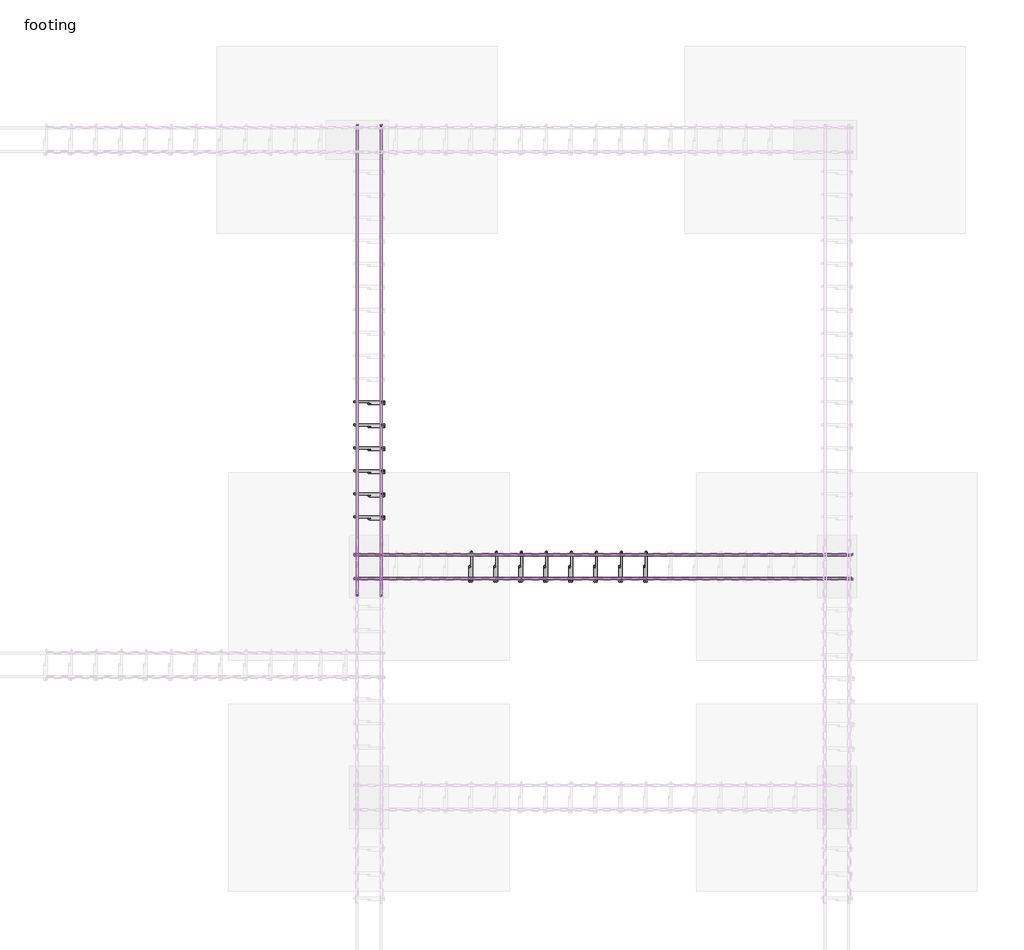
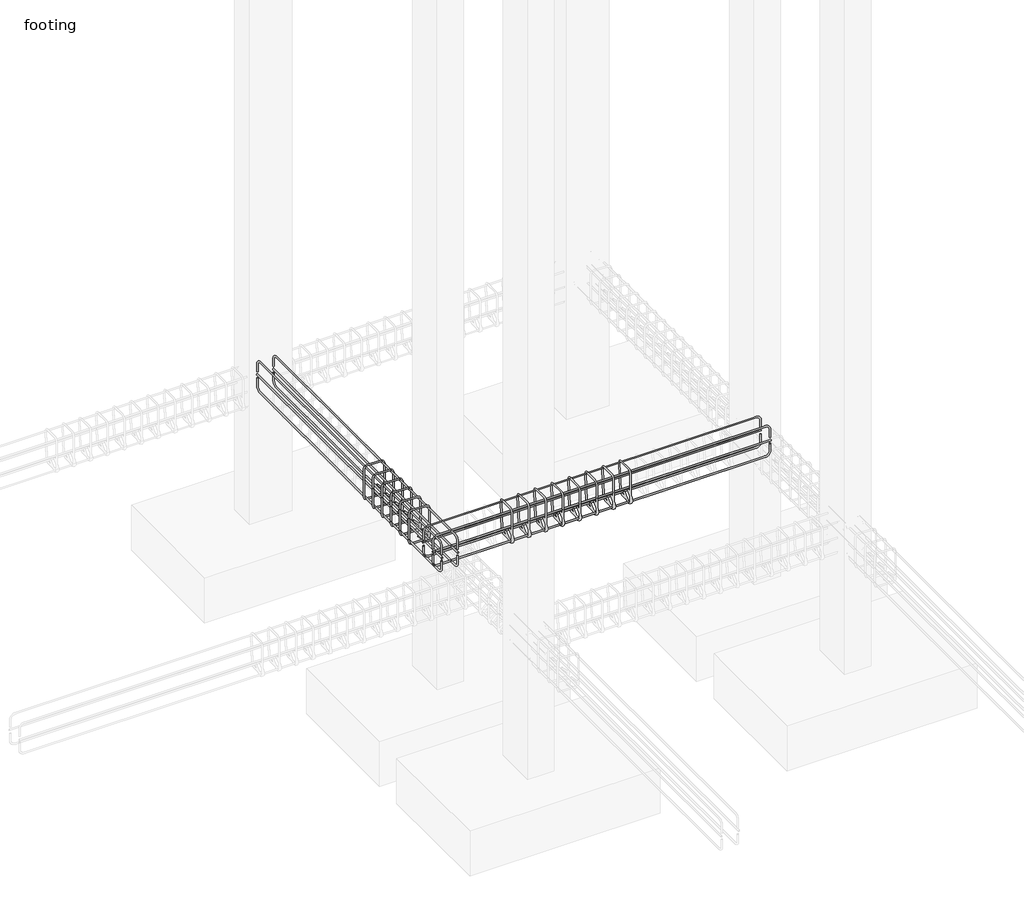
# One storey, part 18 of 21: 27 reinforcing bars.
"""IFC4 building model written with IfcOpenShell, lengths in millimetres."""

from ifc_helpers import new_model, si_unit, point, frame, origin, place, context, project, spatial, polyline, circle_curve, trimmed, segment, composite_curve, element, save
from ifc_brep_helpers import swept_disk

model = new_model("IFC4")

# Units and contexts
model_context = context("Model", 3, world=origin())
ifc_project = project(units=[si_unit("LENGTHUNIT", "METRE", prefix="MILLI")], contexts=[model_context])

# Site, building, storey
site = spatial("IfcSite", under=ifc_project)
building = spatial("IfcBuilding", under=site)
storey = spatial("IfcBuildingStorey", under=building, Name="footing", Elevation=-1524.0)

# Reinforcing bars
placement = place(None, origin())
element("IfcReinforcingBar", 1, at=placement, inside=storey, context=model_context, shape_type="SolidModel", body=[
    swept_disk(composite_curve([segment(polyline([(-4722.5521673, 8277.5872086, -236.1172592), (-4722.5521673, 8277.5872086, -312.3172592)]), True, "CONTINUOUS"), segment(trimmed(circle_curve(frame((-4767.0021673, 8277.5872086, -312.3172592), z_axis=(0.0, 1.0, -2.1166279873208456e-12), x_axis=(44.44999999999982, 0.0, 0.0)), 44.45), [point((-4722.5521673, 8277.5872086, -312.3172592))], [point((-4767.0021673, 8277.5872086, -356.7672592))], True, "CARTESIAN"), True, "CONTINUOUS"), segment(polyline([(-4767.0021673, 8277.5872086, -356.7672592), (-7917.3959173, 8277.5872086, -356.7672592)]), True, "CONTINUOUS"), segment(trimmed(circle_curve(frame((-7917.3959173, 8277.5872086, -312.3172592), z_axis=(0.0, 1.0, -2.1166279873208456e-12), x_axis=(0.0, 0.0, -44.44999999999999)), 44.45), [point((-7917.3959173, 8277.5872086, -356.7672592))], [point((-7961.8459173, 8277.5872086, -312.3172592))], True, "CARTESIAN"), True, "CONTINUOUS"), segment(polyline([(-7961.8459173, 8277.5872086, -312.3172592), (-7961.8459173, 8277.5872086, -236.1172592)]), True, "CONTINUOUS")], self_intersect=False), 6.35),
])
element("IfcReinforcingBar", 2, at=placement, inside=storey, context=model_context, shape_type="SolidModel", body=[
    swept_disk(composite_curve([segment(polyline([(-4722.5521673, 8122.8526902, -170.2827408), (-4722.5521673, 8122.8526902, -94.0827408)]), True, "CONTINUOUS"), segment(trimmed(circle_curve(frame((-4767.0021673, 8122.8526902, -94.0827408), z_axis=(0.0, -1.0, 0.0), x_axis=(44.44999999999982, 0.0, 0.0)), 44.45), [point((-4722.5521673, 8122.8526902, -94.0827408))], [point((-4767.0021673, 8122.8526902, -49.6327408))], True, "CARTESIAN"), True, "CONTINUOUS"), segment(polyline([(-4767.0021673, 8122.8526902, -49.6327408), (-7917.3959173, 8122.8526902, -49.6327408)]), True, "CONTINUOUS"), segment(trimmed(circle_curve(frame((-7917.3959173, 8122.8526902, -94.0827408), z_axis=(0.0, -1.0, 0.0), x_axis=(0.0, 0.0, 44.449999999999996)), 44.45), [point((-7917.3959173, 8122.8526902, -49.6327408))], [point((-7961.8459173, 8122.8526902, -94.0827408))], True, "CARTESIAN"), True, "CONTINUOUS"), segment(polyline([(-7961.8459173, 8122.8526902, -94.0827408), (-7961.8459173, 8122.8526902, -170.2827408)]), True, "CONTINUOUS")], self_intersect=False), 6.35),
])
element("IfcReinforcingBar", 3, at=placement, inside=storey, context=model_context, shape_type="SolidModel", body=[
    swept_disk(composite_curve([segment(polyline([(-4722.5521673, 8122.8526902, -236.1172592), (-4722.5521673, 8122.8526902, -312.3172592)]), True, "CONTINUOUS"), segment(trimmed(circle_curve(frame((-4767.0021673, 8122.8526902, -312.3172592), z_axis=(0.0, 1.0, 2.1166279873208456e-12), x_axis=(44.44999999999982, 0.0, 0.0)), 44.45), [point((-4722.5521673, 8122.8526902, -312.3172592))], [point((-4767.0021673, 8122.8526902, -356.7672592))], True, "CARTESIAN"), True, "CONTINUOUS"), segment(polyline([(-4767.0021673, 8122.8526902, -356.7672592), (-7917.3959173, 8122.8526902, -356.7672592)]), True, "CONTINUOUS"), segment(trimmed(circle_curve(frame((-7917.3959173, 8122.8526902, -312.3172592), z_axis=(0.0, 1.0, 2.1166279873208456e-12), x_axis=(0.0, 0.0, -44.44999999999999)), 44.45), [point((-7917.3959173, 8122.8526902, -356.7672592))], [point((-7961.8459173, 8122.8526902, -312.3172592))], True, "CARTESIAN"), True, "CONTINUOUS"), segment(polyline([(-7961.8459173, 8122.8526902, -312.3172592), (-7961.8459173, 8122.8526902, -236.1172592)]), True, "CONTINUOUS")], self_intersect=False), 6.35),
])
element("IfcReinforcingBar", 4, at=placement, inside=storey, context=model_context, shape_type="SolidModel", body=[
    swept_disk(composite_curve([segment(polyline([(-4722.5521673, 8277.5872086, -170.2827408), (-4722.5521673, 8277.5872086, -94.0827408)]), True, "CONTINUOUS"), segment(trimmed(circle_curve(frame((-4767.0021673, 8277.5872086, -94.0827408), z_axis=(0.0, -1.0, 0.0), x_axis=(44.44999999999982, 0.0, 0.0)), 44.45), [point((-4722.5521673, 8277.5872086, -94.0827408))], [point((-4767.0021673, 8277.5872086, -49.6327408))], True, "CARTESIAN"), True, "CONTINUOUS"), segment(polyline([(-4767.0021673, 8277.5872086, -49.6327408), (-7917.3959173, 8277.5872086, -49.6327408)]), True, "CONTINUOUS"), segment(trimmed(circle_curve(frame((-7917.3959173, 8277.5872086, -94.0827408), z_axis=(0.0, -1.0, 0.0), x_axis=(0.0, 0.0, 44.449999999999996)), 44.45), [point((-7917.3959173, 8277.5872086, -49.6327408))], [point((-7961.8459173, 8277.5872086, -94.0827408))], True, "CARTESIAN"), True, "CONTINUOUS"), segment(polyline([(-7961.8459173, 8277.5872086, -94.0827408), (-7961.8459173, 8277.5872086, -170.2827408)]), True, "CONTINUOUS")], self_intersect=False), 6.35),
])
element("IfcReinforcingBar", 5, at=placement, inside=storey, context=model_context, shape_type="SolidModel", body=[
    swept_disk(composite_curve([segment(polyline([(-4716.2021673, 8283.1668244, -203.2), (-7968.1959173, 8283.1668244, -203.2)]), True, "CONTINUOUS")], self_intersect=False), 6.35),
])
element("IfcReinforcingBar", 6, at=placement, inside=storey, context=model_context, shape_type="SolidModel", body=[
    swept_disk(composite_curve([segment(polyline([(-4716.2021673, 8117.2730744, -203.2), (-7968.1959173, 8117.2730744, -203.2)]), True, "CONTINUOUS")], self_intersect=False), 6.35),
])
element("IfcReinforcingBar", 7, at=placement, inside=storey, context=model_context, shape_type="SolidModel", body=[
    swept_disk(composite_curve([segment(polyline([(-7211.6883428, 8213.6387132, -310.8825168), (-7211.6883428, 8158.7737147, -365.7475153)]), True, "CONTINUOUS"), segment(trimmed(circle_curve(frame((-7211.6883428, 8136.3230744, -343.296875), z_axis=(-1.0, 0.0, 0.0), x_axis=(0.0, 22.450640299999577, -22.450640299999975)), 31.75), [point((-7211.6883428, 8158.7737147, -365.7475153))], [point((-7211.6883428, 8104.5730744, -343.296875))], True, "CARTESIAN"), True, "CONTINUOUS"), segment(polyline([(-7211.6883428, 8104.5730744, -343.296875), (-7211.6883428, 8104.5730744, -63.103125)]), True, "CONTINUOUS"), segment(trimmed(circle_curve(frame((-7211.6883428, 8136.3230744, -63.103125), z_axis=(-1.0, 0.0, 0.0), x_axis=(0.0, -31.75, 0.0)), 31.75), [point((-7211.6883428, 8104.5730744, -63.103125))], [point((-7211.6883428, 8136.3230744, -31.353125))], True, "CARTESIAN"), True, "CONTINUOUS"), segment(polyline([(-7211.6883428, 8136.3230744, -31.353125), (-7211.6883428, 8264.1168244, -31.353125)]), True, "CONTINUOUS"), segment(trimmed(circle_curve(frame((-7210.5159328, 8264.1168244, -63.0814712), z_axis=(-0.9993179916193466, 0.0, -0.03692629992126919), x_axis=(-1.1724100000001272, 0.0, 31.728346200000004)), 31.75), [point((-7211.6883428, 8264.1168244, -31.353125))], [point((-7210.5159328, 8295.8668244, -63.0814712))], True, "CARTESIAN"), True, "CONTINUOUS"), segment(polyline([(-7210.5159328, 8295.8668244, -63.0814712), (-7200.1607528, 8295.8668244, -343.3185288)]), True, "CONTINUOUS"), segment(trimmed(circle_curve(frame((-7200.1607528, 8264.1168244, -343.3185288), z_axis=(-0.9993179916193466, 0.0, -0.03692629992126919), x_axis=(0.0, 31.75, 0.0)), 31.75), [point((-7200.1607528, 8295.8668244, -343.3185288))], [point((-7198.9883428, 8264.1168244, -375.046875))], True, "CARTESIAN"), True, "CONTINUOUS"), segment(polyline([(-7198.9883428, 8264.1168244, -375.046875), (-7198.9883428, 8136.3230744, -375.046875)]), True, "CONTINUOUS"), segment(trimmed(circle_curve(frame((-7198.9883428, 8136.3230744, -343.296875), z_axis=(-1.0, 0.0, 0.0), x_axis=(0.0, 0.0, -31.75)), 31.75), [point((-7198.9883428, 8136.3230744, -375.046875))], [point((-7198.9883428, 8113.8724341, -320.8462347))], True, "CARTESIAN"), True, "CONTINUOUS"), segment(polyline([(-7198.9883428, 8113.8724341, -320.8462347), (-7198.9883428, 8168.7374326, -265.9812362)]), True, "CONTINUOUS")], self_intersect=False), 6.35),
])
element("IfcReinforcingBar", 8, at=placement, inside=storey, context=model_context, shape_type="SolidModel", body=[
    swept_disk(composite_curve([segment(polyline([(-7048.9883428, 8213.6387132, -310.8825168), (-7048.9883428, 8158.7737147, -365.7475153)]), True, "CONTINUOUS"), segment(trimmed(circle_curve(frame((-7048.9883428, 8136.3230744, -343.296875), z_axis=(-1.0, 0.0, 0.0), x_axis=(0.0, 22.450640299999577, -22.450640299999975)), 31.75), [point((-7048.9883428, 8158.7737147, -365.7475153))], [point((-7048.9883428, 8104.5730744, -343.296875))], True, "CARTESIAN"), True, "CONTINUOUS"), segment(polyline([(-7048.9883428, 8104.5730744, -343.296875), (-7048.9883428, 8104.5730744, -63.103125)]), True, "CONTINUOUS"), segment(trimmed(circle_curve(frame((-7048.9883428, 8136.3230744, -63.103125), z_axis=(-1.0, 0.0, 0.0), x_axis=(0.0, -31.75, 0.0)), 31.75), [point((-7048.9883428, 8104.5730744, -63.103125))], [point((-7048.9883428, 8136.3230744, -31.353125))], True, "CARTESIAN"), True, "CONTINUOUS"), segment(polyline([(-7048.9883428, 8136.3230744, -31.353125), (-7048.9883428, 8264.1168244, -31.353125)]), True, "CONTINUOUS"), segment(trimmed(circle_curve(frame((-7047.8159328, 8264.1168244, -63.0814712), z_axis=(-0.9993179916193466, 0.0, -0.03692629992126919), x_axis=(-1.1724100000001272, 0.0, 31.728346200000004)), 31.75), [point((-7048.9883428, 8264.1168244, -31.353125))], [point((-7047.8159328, 8295.8668244, -63.0814712))], True, "CARTESIAN"), True, "CONTINUOUS"), segment(polyline([(-7047.8159328, 8295.8668244, -63.0814712), (-7037.4607528, 8295.8668244, -343.3185288)]), True, "CONTINUOUS"), segment(trimmed(circle_curve(frame((-7037.4607528, 8264.1168244, -343.3185288), z_axis=(-0.9993179916193466, 0.0, -0.03692629992126919), x_axis=(0.0, 31.75, 0.0)), 31.75), [point((-7037.4607528, 8295.8668244, -343.3185288))], [point((-7036.2883428, 8264.1168244, -375.046875))], True, "CARTESIAN"), True, "CONTINUOUS"), segment(polyline([(-7036.2883428, 8264.1168244, -375.046875), (-7036.2883428, 8136.3230744, -375.046875)]), True, "CONTINUOUS"), segment(trimmed(circle_curve(frame((-7036.2883428, 8136.3230744, -343.296875), z_axis=(-1.0, 0.0, 0.0), x_axis=(0.0, 0.0, -31.75)), 31.75), [point((-7036.2883428, 8136.3230744, -375.046875))], [point((-7036.2883428, 8113.8724341, -320.8462347))], True, "CARTESIAN"), True, "CONTINUOUS"), segment(polyline([(-7036.2883428, 8113.8724341, -320.8462347), (-7036.2883428, 8168.7374326, -265.9812362)]), True, "CONTINUOUS")], self_intersect=False), 6.35),
])
element("IfcReinforcingBar", 9, at=placement, inside=storey, context=model_context, shape_type="SolidModel", body=[
    swept_disk(composite_curve([segment(polyline([(-6886.2883428, 8213.6387132, -310.8825168), (-6886.2883428, 8158.7737147, -365.7475153)]), True, "CONTINUOUS"), segment(trimmed(circle_curve(frame((-6886.2883428, 8136.3230744, -343.296875), z_axis=(-1.0, 0.0, 0.0), x_axis=(0.0, 22.450640299999577, -22.450640299999975)), 31.75), [point((-6886.2883428, 8158.7737147, -365.7475153))], [point((-6886.2883428, 8104.5730744, -343.296875))], True, "CARTESIAN"), True, "CONTINUOUS"), segment(polyline([(-6886.2883428, 8104.5730744, -343.296875), (-6886.2883428, 8104.5730744, -63.103125)]), True, "CONTINUOUS"), segment(trimmed(circle_curve(frame((-6886.2883428, 8136.3230744, -63.103125), z_axis=(-1.0, 0.0, 0.0), x_axis=(0.0, -31.75, 0.0)), 31.75), [point((-6886.2883428, 8104.5730744, -63.103125))], [point((-6886.2883428, 8136.3230744, -31.353125))], True, "CARTESIAN"), True, "CONTINUOUS"), segment(polyline([(-6886.2883428, 8136.3230744, -31.353125), (-6886.2883428, 8264.1168244, -31.353125)]), True, "CONTINUOUS"), segment(trimmed(circle_curve(frame((-6885.1159328, 8264.1168244, -63.0814712), z_axis=(-0.9993179916193466, 0.0, -0.03692629992126919), x_axis=(-1.1724099999992177, 0.0, 31.728346200000004)), 31.75), [point((-6886.2883428, 8264.1168244, -31.353125))], [point((-6885.1159328, 8295.8668244, -63.0814712))], True, "CARTESIAN"), True, "CONTINUOUS"), segment(polyline([(-6885.1159328, 8295.8668244, -63.0814712), (-6874.7607528, 8295.8668244, -343.3185288)]), True, "CONTINUOUS"), segment(trimmed(circle_curve(frame((-6874.7607528, 8264.1168244, -343.3185288), z_axis=(-0.9993179916193466, 0.0, -0.03692629992126919), x_axis=(0.0, 31.75, 0.0)), 31.75), [point((-6874.7607528, 8295.8668244, -343.3185288))], [point((-6873.5883428, 8264.1168244, -375.046875))], True, "CARTESIAN"), True, "CONTINUOUS"), segment(polyline([(-6873.5883428, 8264.1168244, -375.046875), (-6873.5883428, 8136.3230744, -375.046875)]), True, "CONTINUOUS"), segment(trimmed(circle_curve(frame((-6873.5883428, 8136.3230744, -343.296875), z_axis=(-1.0, 0.0, 0.0), x_axis=(0.0, 0.0, -31.75)), 31.75), [point((-6873.5883428, 8136.3230744, -375.046875))], [point((-6873.5883428, 8113.8724341, -320.8462347))], True, "CARTESIAN"), True, "CONTINUOUS"), segment(polyline([(-6873.5883428, 8113.8724341, -320.8462347), (-6873.5883428, 8168.7374326, -265.9812362)]), True, "CONTINUOUS")], self_intersect=False), 6.35),
])
element("IfcReinforcingBar", 10, at=placement, inside=storey, context=model_context, shape_type="SolidModel", body=[
    swept_disk(composite_curve([segment(polyline([(-6723.5883428, 8213.6387132, -310.8825168), (-6723.5883428, 8158.7737147, -365.7475153)]), True, "CONTINUOUS"), segment(trimmed(circle_curve(frame((-6723.5883428, 8136.3230744, -343.296875), z_axis=(-1.0, 0.0, 0.0), x_axis=(0.0, 22.450640299999577, -22.450640299999975)), 31.75), [point((-6723.5883428, 8158.7737147, -365.7475153))], [point((-6723.5883428, 8104.5730744, -343.296875))], True, "CARTESIAN"), True, "CONTINUOUS"), segment(polyline([(-6723.5883428, 8104.5730744, -343.296875), (-6723.5883428, 8104.5730744, -63.103125)]), True, "CONTINUOUS"), segment(trimmed(circle_curve(frame((-6723.5883428, 8136.3230744, -63.103125), z_axis=(-1.0, 0.0, 0.0), x_axis=(0.0, -31.75, 0.0)), 31.75), [point((-6723.5883428, 8104.5730744, -63.103125))], [point((-6723.5883428, 8136.3230744, -31.353125))], True, "CARTESIAN"), True, "CONTINUOUS"), segment(polyline([(-6723.5883428, 8136.3230744, -31.353125), (-6723.5883428, 8264.1168244, -31.353125)]), True, "CONTINUOUS"), segment(trimmed(circle_curve(frame((-6722.4159328, 8264.1168244, -63.0814712), z_axis=(-0.9993179916193466, 0.0, -0.03692629992126919), x_axis=(-1.1724100000001272, 0.0, 31.728346200000004)), 31.75), [point((-6723.5883428, 8264.1168244, -31.353125))], [point((-6722.4159328, 8295.8668244, -63.0814712))], True, "CARTESIAN"), True, "CONTINUOUS"), segment(polyline([(-6722.4159328, 8295.8668244, -63.0814712), (-6712.0607528, 8295.8668244, -343.3185288)]), True, "CONTINUOUS"), segment(trimmed(circle_curve(frame((-6712.0607528, 8264.1168244, -343.3185288), z_axis=(-0.9993179916193466, 0.0, -0.03692629992126919), x_axis=(0.0, 31.75, 0.0)), 31.75), [point((-6712.0607528, 8295.8668244, -343.3185288))], [point((-6710.8883428, 8264.1168244, -375.046875))], True, "CARTESIAN"), True, "CONTINUOUS"), segment(polyline([(-6710.8883428, 8264.1168244, -375.046875), (-6710.8883428, 8136.3230744, -375.046875)]), True, "CONTINUOUS"), segment(trimmed(circle_curve(frame((-6710.8883428, 8136.3230744, -343.296875), z_axis=(-1.0, 0.0, 0.0), x_axis=(0.0, 0.0, -31.75)), 31.75), [point((-6710.8883428, 8136.3230744, -375.046875))], [point((-6710.8883428, 8113.8724341, -320.8462347))], True, "CARTESIAN"), True, "CONTINUOUS"), segment(polyline([(-6710.8883428, 8113.8724341, -320.8462347), (-6710.8883428, 8168.7374326, -265.9812362)]), True, "CONTINUOUS")], self_intersect=False), 6.35),
])
element("IfcReinforcingBar", 11, at=placement, inside=storey, context=model_context, shape_type="SolidModel", body=[
    swept_disk(composite_curve([segment(polyline([(-6560.8883428, 8213.6387132, -310.8825168), (-6560.8883428, 8158.7737147, -365.7475153)]), True, "CONTINUOUS"), segment(trimmed(circle_curve(frame((-6560.8883428, 8136.3230744, -343.296875), z_axis=(-1.0, 0.0, 0.0), x_axis=(0.0, 22.450640299999577, -22.450640299999975)), 31.75), [point((-6560.8883428, 8158.7737147, -365.7475153))], [point((-6560.8883428, 8104.5730744, -343.296875))], True, "CARTESIAN"), True, "CONTINUOUS"), segment(polyline([(-6560.8883428, 8104.5730744, -343.296875), (-6560.8883428, 8104.5730744, -63.103125)]), True, "CONTINUOUS"), segment(trimmed(circle_curve(frame((-6560.8883428, 8136.3230744, -63.103125), z_axis=(-1.0, 0.0, 0.0), x_axis=(0.0, -31.75, 0.0)), 31.75), [point((-6560.8883428, 8104.5730744, -63.103125))], [point((-6560.8883428, 8136.3230744, -31.353125))], True, "CARTESIAN"), True, "CONTINUOUS"), segment(polyline([(-6560.8883428, 8136.3230744, -31.353125), (-6560.8883428, 8264.1168244, -31.353125)]), True, "CONTINUOUS"), segment(trimmed(circle_curve(frame((-6559.7159328, 8264.1168244, -63.0814712), z_axis=(-0.9993179916193466, 0.0, -0.03692629992126919), x_axis=(-1.1724100000001272, 0.0, 31.728346200000004)), 31.75), [point((-6560.8883428, 8264.1168244, -31.353125))], [point((-6559.7159328, 8295.8668244, -63.0814712))], True, "CARTESIAN"), True, "CONTINUOUS"), segment(polyline([(-6559.7159328, 8295.8668244, -63.0814712), (-6549.3607528, 8295.8668244, -343.3185288)]), True, "CONTINUOUS"), segment(trimmed(circle_curve(frame((-6549.3607528, 8264.1168244, -343.3185288), z_axis=(-0.9993179916193466, 0.0, -0.03692629992126919), x_axis=(0.0, 31.75, 0.0)), 31.75), [point((-6549.3607528, 8295.8668244, -343.3185288))], [point((-6548.1883428, 8264.1168244, -375.046875))], True, "CARTESIAN"), True, "CONTINUOUS"), segment(polyline([(-6548.1883428, 8264.1168244, -375.046875), (-6548.1883428, 8136.3230744, -375.046875)]), True, "CONTINUOUS"), segment(trimmed(circle_curve(frame((-6548.1883428, 8136.3230744, -343.296875), z_axis=(-1.0, 0.0, 0.0), x_axis=(0.0, 0.0, -31.75)), 31.75), [point((-6548.1883428, 8136.3230744, -375.046875))], [point((-6548.1883428, 8113.8724341, -320.8462347))], True, "CARTESIAN"), True, "CONTINUOUS"), segment(polyline([(-6548.1883428, 8113.8724341, -320.8462347), (-6548.1883428, 8168.7374326, -265.9812362)]), True, "CONTINUOUS")], self_intersect=False), 6.35),
])
element("IfcReinforcingBar", 12, at=placement, inside=storey, context=model_context, shape_type="SolidModel", body=[
    swept_disk(composite_curve([segment(polyline([(-6398.1883428, 8213.6387132, -310.8825168), (-6398.1883428, 8158.7737147, -365.7475153)]), True, "CONTINUOUS"), segment(trimmed(circle_curve(frame((-6398.1883428, 8136.3230744, -343.296875), z_axis=(-1.0, 0.0, 0.0), x_axis=(0.0, 22.450640299999577, -22.450640299999975)), 31.75), [point((-6398.1883428, 8158.7737147, -365.7475153))], [point((-6398.1883428, 8104.5730744, -343.296875))], True, "CARTESIAN"), True, "CONTINUOUS"), segment(polyline([(-6398.1883428, 8104.5730744, -343.296875), (-6398.1883428, 8104.5730744, -63.103125)]), True, "CONTINUOUS"), segment(trimmed(circle_curve(frame((-6398.1883428, 8136.3230744, -63.103125), z_axis=(-1.0, 0.0, 0.0), x_axis=(0.0, -31.75, 0.0)), 31.75), [point((-6398.1883428, 8104.5730744, -63.103125))], [point((-6398.1883428, 8136.3230744, -31.353125))], True, "CARTESIAN"), True, "CONTINUOUS"), segment(polyline([(-6398.1883428, 8136.3230744, -31.353125), (-6398.1883428, 8264.1168244, -31.353125)]), True, "CONTINUOUS"), segment(trimmed(circle_curve(frame((-6397.0159328, 8264.1168244, -63.0814712), z_axis=(-0.9993179916193466, 0.0, -0.03692629992126919), x_axis=(-1.1724100000001272, 0.0, 31.728346200000004)), 31.75), [point((-6398.1883428, 8264.1168244, -31.353125))], [point((-6397.0159328, 8295.8668244, -63.0814712))], True, "CARTESIAN"), True, "CONTINUOUS"), segment(polyline([(-6397.0159328, 8295.8668244, -63.0814712), (-6386.6607528, 8295.8668244, -343.3185288)]), True, "CONTINUOUS"), segment(trimmed(circle_curve(frame((-6386.6607528, 8264.1168244, -343.3185288), z_axis=(-0.9993179916193466, 0.0, -0.03692629992126919), x_axis=(0.0, 31.75, 0.0)), 31.75), [point((-6386.6607528, 8295.8668244, -343.3185288))], [point((-6385.4883428, 8264.1168244, -375.046875))], True, "CARTESIAN"), True, "CONTINUOUS"), segment(polyline([(-6385.4883428, 8264.1168244, -375.046875), (-6385.4883428, 8136.3230744, -375.046875)]), True, "CONTINUOUS"), segment(trimmed(circle_curve(frame((-6385.4883428, 8136.3230744, -343.296875), z_axis=(-1.0, 0.0, 0.0), x_axis=(0.0, 0.0, -31.75)), 31.75), [point((-6385.4883428, 8136.3230744, -375.046875))], [point((-6385.4883428, 8113.8724341, -320.8462347))], True, "CARTESIAN"), True, "CONTINUOUS"), segment(polyline([(-6385.4883428, 8113.8724341, -320.8462347), (-6385.4883428, 8168.7374326, -265.9812362)]), True, "CONTINUOUS")], self_intersect=False), 6.35),
])
element("IfcReinforcingBar", 13, at=placement, inside=storey, context=model_context, shape_type="SolidModel", body=[
    swept_disk(composite_curve([segment(polyline([(-6235.4883428, 8213.6387132, -310.8825168), (-6235.4883428, 8158.7737147, -365.7475153)]), True, "CONTINUOUS"), segment(trimmed(circle_curve(frame((-6235.4883428, 8136.3230744, -343.296875), z_axis=(-1.0, 0.0, 0.0), x_axis=(0.0, 22.450640299999577, -22.450640299999975)), 31.75), [point((-6235.4883428, 8158.7737147, -365.7475153))], [point((-6235.4883428, 8104.5730744, -343.296875))], True, "CARTESIAN"), True, "CONTINUOUS"), segment(polyline([(-6235.4883428, 8104.5730744, -343.296875), (-6235.4883428, 8104.5730744, -63.103125)]), True, "CONTINUOUS"), segment(trimmed(circle_curve(frame((-6235.4883428, 8136.3230744, -63.103125), z_axis=(-1.0, 0.0, 0.0), x_axis=(0.0, -31.75, 0.0)), 31.75), [point((-6235.4883428, 8104.5730744, -63.103125))], [point((-6235.4883428, 8136.3230744, -31.353125))], True, "CARTESIAN"), True, "CONTINUOUS"), segment(polyline([(-6235.4883428, 8136.3230744, -31.353125), (-6235.4883428, 8264.1168244, -31.353125)]), True, "CONTINUOUS"), segment(trimmed(circle_curve(frame((-6234.3159328, 8264.1168244, -63.0814712), z_axis=(-0.9993179916193466, 0.0, -0.03692629992126919), x_axis=(-1.1724100000001272, 0.0, 31.728346200000004)), 31.75), [point((-6235.4883428, 8264.1168244, -31.353125))], [point((-6234.3159328, 8295.8668244, -63.0814712))], True, "CARTESIAN"), True, "CONTINUOUS"), segment(polyline([(-6234.3159328, 8295.8668244, -63.0814712), (-6223.9607528, 8295.8668244, -343.3185288)]), True, "CONTINUOUS"), segment(trimmed(circle_curve(frame((-6223.9607528, 8264.1168244, -343.3185288), z_axis=(-0.9993179916193466, 0.0, -0.03692629992126919), x_axis=(0.0, 31.75, 0.0)), 31.75), [point((-6223.9607528, 8295.8668244, -343.3185288))], [point((-6222.7883428, 8264.1168244, -375.046875))], True, "CARTESIAN"), True, "CONTINUOUS"), segment(polyline([(-6222.7883428, 8264.1168244, -375.046875), (-6222.7883428, 8136.3230744, -375.046875)]), True, "CONTINUOUS"), segment(trimmed(circle_curve(frame((-6222.7883428, 8136.3230744, -343.296875), z_axis=(-1.0, 0.0, 0.0), x_axis=(0.0, 0.0, -31.75)), 31.75), [point((-6222.7883428, 8136.3230744, -375.046875))], [point((-6222.7883428, 8113.8724341, -320.8462347))], True, "CARTESIAN"), True, "CONTINUOUS"), segment(polyline([(-6222.7883428, 8113.8724341, -320.8462347), (-6222.7883428, 8168.7374326, -265.9812362)]), True, "CONTINUOUS")], self_intersect=False), 6.35),
])
element("IfcReinforcingBar", 14, at=placement, inside=storey, context=model_context, shape_type="SolidModel", body=[
    swept_disk(composite_curve([segment(polyline([(-6072.7883428, 8213.6387132, -310.8825168), (-6072.7883428, 8158.7737147, -365.7475153)]), True, "CONTINUOUS"), segment(trimmed(circle_curve(frame((-6072.7883428, 8136.3230744, -343.296875), z_axis=(-1.0, 0.0, 0.0), x_axis=(0.0, 22.450640299999577, -22.450640299999975)), 31.75), [point((-6072.7883428, 8158.7737147, -365.7475153))], [point((-6072.7883428, 8104.5730744, -343.296875))], True, "CARTESIAN"), True, "CONTINUOUS"), segment(polyline([(-6072.7883428, 8104.5730744, -343.296875), (-6072.7883428, 8104.5730744, -63.103125)]), True, "CONTINUOUS"), segment(trimmed(circle_curve(frame((-6072.7883428, 8136.3230744, -63.103125), z_axis=(-1.0, 0.0, 0.0), x_axis=(0.0, -31.75, 0.0)), 31.75), [point((-6072.7883428, 8104.5730744, -63.103125))], [point((-6072.7883428, 8136.3230744, -31.353125))], True, "CARTESIAN"), True, "CONTINUOUS"), segment(polyline([(-6072.7883428, 8136.3230744, -31.353125), (-6072.7883428, 8264.1168244, -31.353125)]), True, "CONTINUOUS"), segment(trimmed(circle_curve(frame((-6071.6159328, 8264.1168244, -63.0814712), z_axis=(-0.9993179916193466, 0.0, -0.03692629992126919), x_axis=(-1.1724099999992177, 0.0, 31.728346200000004)), 31.75), [point((-6072.7883428, 8264.1168244, -31.353125))], [point((-6071.6159328, 8295.8668244, -63.0814712))], True, "CARTESIAN"), True, "CONTINUOUS"), segment(polyline([(-6071.6159328, 8295.8668244, -63.0814712), (-6061.2607528, 8295.8668244, -343.3185288)]), True, "CONTINUOUS"), segment(trimmed(circle_curve(frame((-6061.2607528, 8264.1168244, -343.3185288), z_axis=(-0.9993179916193466, 0.0, -0.03692629992126919), x_axis=(0.0, 31.75, 0.0)), 31.75), [point((-6061.2607528, 8295.8668244, -343.3185288))], [point((-6060.0883428, 8264.1168244, -375.046875))], True, "CARTESIAN"), True, "CONTINUOUS"), segment(polyline([(-6060.0883428, 8264.1168244, -375.046875), (-6060.0883428, 8136.3230744, -375.046875)]), True, "CONTINUOUS"), segment(trimmed(circle_curve(frame((-6060.0883428, 8136.3230744, -343.296875), z_axis=(-1.0, 0.0, 0.0), x_axis=(0.0, 0.0, -31.75)), 31.75), [point((-6060.0883428, 8136.3230744, -375.046875))], [point((-6060.0883428, 8113.8724341, -320.8462347))], True, "CARTESIAN"), True, "CONTINUOUS"), segment(polyline([(-6060.0883428, 8113.8724341, -320.8462347), (-6060.0883428, 8168.7374326, -265.9812362)]), True, "CONTINUOUS")], self_intersect=False), 6.35),
])
element("IfcReinforcingBar", 15, at=placement, inside=storey, context=model_context, shape_type="SolidModel", body=[
    swept_disk(composite_curve([segment(polyline([(-7834.7165254, 8525.2699494, -265.9812362), (-7779.851527, 8525.2699494, -320.8462347)]), True, "CONTINUOUS"), segment(trimmed(circle_curve(frame((-7802.3021673, 8525.2699494, -343.296875), z_axis=(0.0, 1.0, 0.0), x_axis=(22.450640300000487, 0.0, 22.450640299999975)), 31.75), [point((-7779.851527, 8525.2699494, -320.8462347))], [point((-7802.3021673, 8525.2699494, -375.046875))], True, "CARTESIAN"), True, "CONTINUOUS"), segment(polyline([(-7802.3021673, 8525.2699494, -375.046875), (-7930.0959173, 8525.2699494, -375.046875)]), True, "CONTINUOUS"), segment(trimmed(circle_curve(frame((-7930.0959173, 8525.2699494, -343.296875), z_axis=(0.0, 1.0, 0.0), x_axis=(0.0, 0.0, -31.75)), 31.75), [point((-7930.0959173, 8525.2699494, -375.046875))], [point((-7961.8459173, 8525.2699494, -343.296875))], True, "CARTESIAN"), True, "CONTINUOUS"), segment(polyline([(-7961.8459173, 8525.2699494, -343.296875), (-7961.8459173, 8525.2699494, -63.103125)]), True, "CONTINUOUS"), segment(trimmed(circle_curve(frame((-7930.165658, 8523.1666957, -63.103125), z_axis=(0.06624421176864137, 0.9978034397651431, 0.0), x_axis=(-31.680259300000216, 2.103253700001005, 0.0)), 31.75), [point((-7961.8459173, 8525.2699494, -63.103125))], [point((-7930.165658, 8523.1666957, -31.353125))], True, "CARTESIAN"), True, "CONTINUOUS"), segment(polyline([(-7930.165658, 8523.1666957, -31.353125), (-7802.2324265, 8514.6732031, -31.353125)]), True, "CONTINUOUS"), segment(trimmed(circle_curve(frame((-7802.2324265, 8514.6732031, -63.103125), z_axis=(0.06624421176864137, 0.9978034397651431, 0.0), x_axis=(0.0, 0.0, 31.75)), 31.75), [point((-7802.2324265, 8514.6732031, -31.353125))], [point((-7770.5521673, 8512.5699494, -63.103125))], True, "CARTESIAN"), True, "CONTINUOUS"), segment(polyline([(-7770.5521673, 8512.5699494, -63.103125), (-7770.5521673, 8512.5699494, -343.296875)]), True, "CONTINUOUS"), segment(trimmed(circle_curve(frame((-7802.3021673, 8512.5699494, -343.296875), z_axis=(0.0, 1.0, 0.0), x_axis=(31.75, 0.0, 0.0)), 31.75), [point((-7770.5521673, 8512.5699494, -343.296875))], [point((-7824.7528076, 8512.5699494, -365.7475153))], True, "CARTESIAN"), True, "CONTINUOUS"), segment(polyline([(-7824.7528076, 8512.5699494, -365.7475153), (-7879.617806, 8512.5699494, -310.8825168)]), True, "CONTINUOUS")], self_intersect=False), 6.35),
])
element("IfcReinforcingBar", 16, at=placement, inside=storey, context=model_context, shape_type="SolidModel", body=[
    swept_disk(composite_curve([segment(polyline([(-7788.8317831, 8012.5359344, -170.2827408), (-7788.8317831, 8012.5359344, -94.0827408)]), True, "CONTINUOUS"), segment(trimmed(circle_curve(frame((-7788.8317831, 8056.9859344, -94.0827408), z_axis=(-1.0, 0.0, 0.0), x_axis=(0.0, -44.44999999999982, 0.0)), 44.45), [point((-7788.8317831, 8012.5359344, -94.0827408))], [point((-7788.8317831, 8056.9859344, -49.6327408))], True, "CARTESIAN"), True, "CONTINUOUS"), segment(polyline([(-7788.8317831, 8056.9859344, -49.6327408), (-7788.8317831, 11032.7168244, -49.6327408)]), True, "CONTINUOUS"), segment(trimmed(circle_curve(frame((-7788.8317831, 11032.7168244, -94.0827408), z_axis=(-1.0, 0.0, 0.0), x_axis=(0.0, 0.0, 44.449999999999996)), 44.45), [point((-7788.8317831, 11032.7168244, -49.6327408))], [point((-7788.8317831, 11077.1668244, -94.0827408))], True, "CARTESIAN"), True, "CONTINUOUS"), segment(polyline([(-7788.8317831, 11077.1668244, -94.0827408), (-7788.8317831, 11077.1668244, -170.2827408)]), True, "CONTINUOUS")], self_intersect=False), 6.35),
])
element("IfcReinforcingBar", 17, at=placement, inside=storey, context=model_context, shape_type="SolidModel", body=[
    swept_disk(composite_curve([segment(polyline([(-7943.5663014, 8012.5359344, -170.2827408), (-7943.5663014, 8012.5359344, -94.0827408)]), True, "CONTINUOUS"), segment(trimmed(circle_curve(frame((-7943.5663014, 8056.9859344, -94.0827408), z_axis=(-1.0, 0.0, 0.0), x_axis=(0.0, -44.44999999999982, 0.0)), 44.45), [point((-7943.5663014, 8012.5359344, -94.0827408))], [point((-7943.5663014, 8056.9859344, -49.6327408))], True, "CARTESIAN"), True, "CONTINUOUS"), segment(polyline([(-7943.5663014, 8056.9859344, -49.6327408), (-7943.5663014, 11032.7168244, -49.6327408)]), True, "CONTINUOUS"), segment(trimmed(circle_curve(frame((-7943.5663014, 11032.7168244, -94.0827408), z_axis=(-1.0, 0.0, 0.0), x_axis=(0.0, 0.0, 44.449999999999996)), 44.45), [point((-7943.5663014, 11032.7168244, -49.6327408))], [point((-7943.5663014, 11077.1668244, -94.0827408))], True, "CARTESIAN"), True, "CONTINUOUS"), segment(polyline([(-7943.5663014, 11077.1668244, -94.0827408), (-7943.5663014, 11077.1668244, -170.2827408)]), True, "CONTINUOUS")], self_intersect=False), 6.35),
])
element("IfcReinforcingBar", 18, at=placement, inside=storey, context=model_context, shape_type="SolidModel", body=[
    swept_disk(composite_curve([segment(polyline([(-7788.8317831, 8012.5359344, -236.1172592), (-7788.8317831, 8012.5359344, -312.3172592)]), True, "CONTINUOUS"), segment(trimmed(circle_curve(frame((-7788.8317831, 8056.9859344, -312.3172592), z_axis=(1.0, 0.0, 0.0), x_axis=(0.0, -44.44999999999982, 0.0)), 44.45), [point((-7788.8317831, 8012.5359344, -312.3172592))], [point((-7788.8317831, 8056.9859344, -356.7672592))], True, "CARTESIAN"), True, "CONTINUOUS"), segment(polyline([(-7788.8317831, 8056.9859344, -356.7672592), (-7788.8317831, 11032.7168244, -356.7672592)]), True, "CONTINUOUS"), segment(trimmed(circle_curve(frame((-7788.8317831, 11032.7168244, -312.3172592), z_axis=(1.0, 0.0, 0.0), x_axis=(0.0, 0.0, -44.44999999999999)), 44.45), [point((-7788.8317831, 11032.7168244, -356.7672592))], [point((-7788.8317831, 11077.1668244, -312.3172592))], True, "CARTESIAN"), True, "CONTINUOUS"), segment(polyline([(-7788.8317831, 11077.1668244, -312.3172592), (-7788.8317831, 11077.1668244, -236.1172592)]), True, "CONTINUOUS")], self_intersect=False), 6.35),
])
element("IfcReinforcingBar", 19, at=placement, inside=storey, context=model_context, shape_type="SolidModel", body=[
    swept_disk(composite_curve([segment(polyline([(-7943.5663014, 8012.5359344, -236.1172592), (-7943.5663014, 8012.5359344, -312.3172592)]), True, "CONTINUOUS"), segment(trimmed(circle_curve(frame((-7943.5663014, 8056.9859344, -312.3172592), z_axis=(1.0, 0.0, 0.0), x_axis=(0.0, -44.44999999999982, 0.0)), 44.45), [point((-7943.5663014, 8012.5359344, -312.3172592))], [point((-7943.5663014, 8056.9859344, -356.7672592))], True, "CARTESIAN"), True, "CONTINUOUS"), segment(polyline([(-7943.5663014, 8056.9859344, -356.7672592), (-7943.5663014, 11032.7168244, -356.7672592)]), True, "CONTINUOUS"), segment(trimmed(circle_curve(frame((-7943.5663014, 11032.7168244, -312.3172592), z_axis=(1.0, 0.0, 0.0), x_axis=(0.0, 0.0, -44.44999999999999)), 44.45), [point((-7943.5663014, 11032.7168244, -356.7672592))], [point((-7943.5663014, 11077.1668244, -312.3172592))], True, "CARTESIAN"), True, "CONTINUOUS"), segment(polyline([(-7943.5663014, 11077.1668244, -312.3172592), (-7943.5663014, 11077.1668244, -236.1172592)]), True, "CONTINUOUS")], self_intersect=False), 6.35),
])
element("IfcReinforcingBar", 20, at=placement, inside=storey, context=model_context, shape_type="SolidModel", body=[
    swept_disk(composite_curve([segment(polyline([(-7943.5663014, 8006.1859344, -203.2), (-7943.5663014, 11083.5168244, -203.2)]), True, "CONTINUOUS")], self_intersect=False), 6.35),
])
element("IfcReinforcingBar", 21, at=placement, inside=storey, context=model_context, shape_type="SolidModel", body=[
    swept_disk(composite_curve([segment(polyline([(-7943.5663014, 8006.1859344, -203.2), (-7943.5663014, 11083.5168244, -203.2)]), True, "CONTINUOUS")], self_intersect=False), 6.35),
])
element("IfcReinforcingBar", 22, at=placement, inside=storey, context=model_context, shape_type="SolidModel", body=[
    swept_disk(composite_curve([segment(polyline([(-7788.8317831, 8006.1859344, -203.2), (-7788.8317831, 11083.5168244, -203.2)]), True, "CONTINUOUS")], self_intersect=False), 6.35),
])
element("IfcReinforcingBar", 23, at=placement, inside=storey, context=model_context, shape_type="SolidModel", body=[
    swept_disk(composite_curve([segment(polyline([(-7834.7165254, 8675.2699494, -265.9812362), (-7779.851527, 8675.2699494, -320.8462347)]), True, "CONTINUOUS"), segment(trimmed(circle_curve(frame((-7802.3021673, 8675.2699494, -343.296875), z_axis=(0.0, 1.0, 0.0), x_axis=(22.450640300000487, 0.0, 22.450640299999975)), 31.75), [point((-7779.851527, 8675.2699494, -320.8462347))], [point((-7802.3021673, 8675.2699494, -375.046875))], True, "CARTESIAN"), True, "CONTINUOUS"), segment(polyline([(-7802.3021673, 8675.2699494, -375.046875), (-7930.0959173, 8675.2699494, -375.046875)]), True, "CONTINUOUS"), segment(trimmed(circle_curve(frame((-7930.0959173, 8675.2699494, -343.296875), z_axis=(0.0, 1.0, 0.0), x_axis=(0.0, 0.0, -31.75)), 31.75), [point((-7930.0959173, 8675.2699494, -375.046875))], [point((-7961.8459173, 8675.2699494, -343.296875))], True, "CARTESIAN"), True, "CONTINUOUS"), segment(polyline([(-7961.8459173, 8675.2699494, -343.296875), (-7961.8459173, 8675.2699494, -63.103125)]), True, "CONTINUOUS"), segment(trimmed(circle_curve(frame((-7930.165658, 8673.1666957, -63.103125), z_axis=(0.06624421176864137, 0.9978034397651431, 0.0), x_axis=(-31.680259300000216, 2.103253700001005, 0.0)), 31.75), [point((-7961.8459173, 8675.2699494, -63.103125))], [point((-7930.165658, 8673.1666957, -31.353125))], True, "CARTESIAN"), True, "CONTINUOUS"), segment(polyline([(-7930.165658, 8673.1666957, -31.353125), (-7802.2324265, 8664.6732031, -31.353125)]), True, "CONTINUOUS"), segment(trimmed(circle_curve(frame((-7802.2324265, 8664.6732031, -63.103125), z_axis=(0.06624421176864137, 0.9978034397651431, 0.0), x_axis=(0.0, 0.0, 31.75)), 31.75), [point((-7802.2324265, 8664.6732031, -31.353125))], [point((-7770.5521673, 8662.5699494, -63.103125))], True, "CARTESIAN"), True, "CONTINUOUS"), segment(polyline([(-7770.5521673, 8662.5699494, -63.103125), (-7770.5521673, 8662.5699494, -343.296875)]), True, "CONTINUOUS"), segment(trimmed(circle_curve(frame((-7802.3021673, 8662.5699494, -343.296875), z_axis=(0.0, 1.0, 0.0), x_axis=(31.75, 0.0, 0.0)), 31.75), [point((-7770.5521673, 8662.5699494, -343.296875))], [point((-7824.7528076, 8662.5699494, -365.7475153))], True, "CARTESIAN"), True, "CONTINUOUS"), segment(polyline([(-7824.7528076, 8662.5699494, -365.7475153), (-7879.617806, 8662.5699494, -310.8825168)]), True, "CONTINUOUS")], self_intersect=False), 6.35),
])
element("IfcReinforcingBar", 24, at=placement, inside=storey, context=model_context, shape_type="SolidModel", body=[
    swept_disk(composite_curve([segment(polyline([(-7834.7165254, 8825.2699494, -265.9812362), (-7779.851527, 8825.2699494, -320.8462347)]), True, "CONTINUOUS"), segment(trimmed(circle_curve(frame((-7802.3021673, 8825.2699494, -343.296875), z_axis=(0.0, 1.0, 0.0), x_axis=(22.450640300000487, 0.0, 22.450640299999975)), 31.75), [point((-7779.851527, 8825.2699494, -320.8462347))], [point((-7802.3021673, 8825.2699494, -375.046875))], True, "CARTESIAN"), True, "CONTINUOUS"), segment(polyline([(-7802.3021673, 8825.2699494, -375.046875), (-7930.0959173, 8825.2699494, -375.046875)]), True, "CONTINUOUS"), segment(trimmed(circle_curve(frame((-7930.0959173, 8825.2699494, -343.296875), z_axis=(0.0, 1.0, 0.0), x_axis=(0.0, 0.0, -31.75)), 31.75), [point((-7930.0959173, 8825.2699494, -375.046875))], [point((-7961.8459173, 8825.2699494, -343.296875))], True, "CARTESIAN"), True, "CONTINUOUS"), segment(polyline([(-7961.8459173, 8825.2699494, -343.296875), (-7961.8459173, 8825.2699494, -63.103125)]), True, "CONTINUOUS"), segment(trimmed(circle_curve(frame((-7930.165658, 8823.1666957, -63.103125), z_axis=(0.06624421176864137, 0.9978034397651431, 0.0), x_axis=(-31.680259300000216, 2.103253700001005, 0.0)), 31.75), [point((-7961.8459173, 8825.2699494, -63.103125))], [point((-7930.165658, 8823.1666957, -31.353125))], True, "CARTESIAN"), True, "CONTINUOUS"), segment(polyline([(-7930.165658, 8823.1666957, -31.353125), (-7802.2324265, 8814.6732031, -31.353125)]), True, "CONTINUOUS"), segment(trimmed(circle_curve(frame((-7802.2324265, 8814.6732031, -63.103125), z_axis=(0.06624421176864137, 0.9978034397651431, 0.0), x_axis=(0.0, 0.0, 31.75)), 31.75), [point((-7802.2324265, 8814.6732031, -31.353125))], [point((-7770.5521673, 8812.5699494, -63.103125))], True, "CARTESIAN"), True, "CONTINUOUS"), segment(polyline([(-7770.5521673, 8812.5699494, -63.103125), (-7770.5521673, 8812.5699494, -343.296875)]), True, "CONTINUOUS"), segment(trimmed(circle_curve(frame((-7802.3021673, 8812.5699494, -343.296875), z_axis=(0.0, 1.0, 0.0), x_axis=(31.75, 0.0, 0.0)), 31.75), [point((-7770.5521673, 8812.5699494, -343.296875))], [point((-7824.7528076, 8812.5699494, -365.7475153))], True, "CARTESIAN"), True, "CONTINUOUS"), segment(polyline([(-7824.7528076, 8812.5699494, -365.7475153), (-7879.617806, 8812.5699494, -310.8825168)]), True, "CONTINUOUS")], self_intersect=False), 6.35),
])
element("IfcReinforcingBar", 25, at=placement, inside=storey, context=model_context, shape_type="SolidModel", body=[
    swept_disk(composite_curve([segment(polyline([(-7834.7165254, 8975.2699494, -265.9812362), (-7779.851527, 8975.2699494, -320.8462347)]), True, "CONTINUOUS"), segment(trimmed(circle_curve(frame((-7802.3021673, 8975.2699494, -343.296875), z_axis=(0.0, 1.0, 0.0), x_axis=(22.450640300000487, 0.0, 22.450640299999975)), 31.75), [point((-7779.851527, 8975.2699494, -320.8462347))], [point((-7802.3021673, 8975.2699494, -375.046875))], True, "CARTESIAN"), True, "CONTINUOUS"), segment(polyline([(-7802.3021673, 8975.2699494, -375.046875), (-7930.0959173, 8975.2699494, -375.046875)]), True, "CONTINUOUS"), segment(trimmed(circle_curve(frame((-7930.0959173, 8975.2699494, -343.296875), z_axis=(0.0, 1.0, 0.0), x_axis=(0.0, 0.0, -31.75)), 31.75), [point((-7930.0959173, 8975.2699494, -375.046875))], [point((-7961.8459173, 8975.2699494, -343.296875))], True, "CARTESIAN"), True, "CONTINUOUS"), segment(polyline([(-7961.8459173, 8975.2699494, -343.296875), (-7961.8459173, 8975.2699494, -63.103125)]), True, "CONTINUOUS"), segment(trimmed(circle_curve(frame((-7930.165658, 8973.1666957, -63.103125), z_axis=(0.06624421176864137, 0.9978034397651431, 0.0), x_axis=(-31.680259300000216, 2.103253700001005, 0.0)), 31.75), [point((-7961.8459173, 8975.2699494, -63.103125))], [point((-7930.165658, 8973.1666957, -31.353125))], True, "CARTESIAN"), True, "CONTINUOUS"), segment(polyline([(-7930.165658, 8973.1666957, -31.353125), (-7802.2324265, 8964.6732031, -31.353125)]), True, "CONTINUOUS"), segment(trimmed(circle_curve(frame((-7802.2324265, 8964.6732031, -63.103125), z_axis=(0.06624421176864137, 0.9978034397651431, 0.0), x_axis=(0.0, 0.0, 31.75)), 31.75), [point((-7802.2324265, 8964.6732031, -31.353125))], [point((-7770.5521673, 8962.5699494, -63.103125))], True, "CARTESIAN"), True, "CONTINUOUS"), segment(polyline([(-7770.5521673, 8962.5699494, -63.103125), (-7770.5521673, 8962.5699494, -343.296875)]), True, "CONTINUOUS"), segment(trimmed(circle_curve(frame((-7802.3021673, 8962.5699494, -343.296875), z_axis=(0.0, 1.0, 0.0), x_axis=(31.75, 0.0, 0.0)), 31.75), [point((-7770.5521673, 8962.5699494, -343.296875))], [point((-7824.7528076, 8962.5699494, -365.7475153))], True, "CARTESIAN"), True, "CONTINUOUS"), segment(polyline([(-7824.7528076, 8962.5699494, -365.7475153), (-7879.617806, 8962.5699494, -310.8825168)]), True, "CONTINUOUS")], self_intersect=False), 6.35),
])
element("IfcReinforcingBar", 26, at=placement, inside=storey, context=model_context, shape_type="SolidModel", body=[
    swept_disk(composite_curve([segment(polyline([(-7834.7165254, 9125.2699494, -265.9812362), (-7779.851527, 9125.2699494, -320.8462347)]), True, "CONTINUOUS"), segment(trimmed(circle_curve(frame((-7802.3021673, 9125.2699494, -343.296875), z_axis=(0.0, 1.0, 0.0), x_axis=(22.450640300000487, 0.0, 22.450640299999975)), 31.75), [point((-7779.851527, 9125.2699494, -320.8462347))], [point((-7802.3021673, 9125.2699494, -375.046875))], True, "CARTESIAN"), True, "CONTINUOUS"), segment(polyline([(-7802.3021673, 9125.2699494, -375.046875), (-7930.0959173, 9125.2699494, -375.046875)]), True, "CONTINUOUS"), segment(trimmed(circle_curve(frame((-7930.0959173, 9125.2699494, -343.296875), z_axis=(0.0, 1.0, 0.0), x_axis=(0.0, 0.0, -31.75)), 31.75), [point((-7930.0959173, 9125.2699494, -375.046875))], [point((-7961.8459173, 9125.2699494, -343.296875))], True, "CARTESIAN"), True, "CONTINUOUS"), segment(polyline([(-7961.8459173, 9125.2699494, -343.296875), (-7961.8459173, 9125.2699494, -63.103125)]), True, "CONTINUOUS"), segment(trimmed(circle_curve(frame((-7930.165658, 9123.1666957, -63.103125), z_axis=(0.06624421176864137, 0.9978034397651431, 0.0), x_axis=(-31.680259300000216, 2.103253700001005, 0.0)), 31.75), [point((-7961.8459173, 9125.2699494, -63.103125))], [point((-7930.165658, 9123.1666957, -31.353125))], True, "CARTESIAN"), True, "CONTINUOUS"), segment(polyline([(-7930.165658, 9123.1666957, -31.353125), (-7802.2324265, 9114.6732031, -31.353125)]), True, "CONTINUOUS"), segment(trimmed(circle_curve(frame((-7802.2324265, 9114.6732031, -63.103125), z_axis=(0.06624421176864137, 0.9978034397651431, 0.0), x_axis=(0.0, 0.0, 31.75)), 31.75), [point((-7802.2324265, 9114.6732031, -31.353125))], [point((-7770.5521673, 9112.5699494, -63.103125))], True, "CARTESIAN"), True, "CONTINUOUS"), segment(polyline([(-7770.5521673, 9112.5699494, -63.103125), (-7770.5521673, 9112.5699494, -343.296875)]), True, "CONTINUOUS"), segment(trimmed(circle_curve(frame((-7802.3021673, 9112.5699494, -343.296875), z_axis=(0.0, 1.0, 0.0), x_axis=(31.75, 0.0, 0.0)), 31.75), [point((-7770.5521673, 9112.5699494, -343.296875))], [point((-7824.7528076, 9112.5699494, -365.7475153))], True, "CARTESIAN"), True, "CONTINUOUS"), segment(polyline([(-7824.7528076, 9112.5699494, -365.7475153), (-7879.617806, 9112.5699494, -310.8825168)]), True, "CONTINUOUS")], self_intersect=False), 6.35),
])
element("IfcReinforcingBar", 27, at=placement, inside=storey, context=model_context, shape_type="SolidModel", body=[
    swept_disk(composite_curve([segment(polyline([(-7834.7165254, 9275.2699494, -265.9812362), (-7779.851527, 9275.2699494, -320.8462347)]), True, "CONTINUOUS"), segment(trimmed(circle_curve(frame((-7802.3021673, 9275.2699494, -343.296875), z_axis=(0.0, 1.0, 0.0), x_axis=(22.450640300000487, 0.0, 22.450640299999975)), 31.75), [point((-7779.851527, 9275.2699494, -320.8462347))], [point((-7802.3021673, 9275.2699494, -375.046875))], True, "CARTESIAN"), True, "CONTINUOUS"), segment(polyline([(-7802.3021673, 9275.2699494, -375.046875), (-7930.0959173, 9275.2699494, -375.046875)]), True, "CONTINUOUS"), segment(trimmed(circle_curve(frame((-7930.0959173, 9275.2699494, -343.296875), z_axis=(0.0, 1.0, 0.0), x_axis=(0.0, 0.0, -31.75)), 31.75), [point((-7930.0959173, 9275.2699494, -375.046875))], [point((-7961.8459173, 9275.2699494, -343.296875))], True, "CARTESIAN"), True, "CONTINUOUS"), segment(polyline([(-7961.8459173, 9275.2699494, -343.296875), (-7961.8459173, 9275.2699494, -63.103125)]), True, "CONTINUOUS"), segment(trimmed(circle_curve(frame((-7930.165658, 9273.1666957, -63.103125), z_axis=(0.06624421176864137, 0.9978034397651431, 0.0), x_axis=(-31.680259300000216, 2.103253700001005, 0.0)), 31.75), [point((-7961.8459173, 9275.2699494, -63.103125))], [point((-7930.165658, 9273.1666957, -31.353125))], True, "CARTESIAN"), True, "CONTINUOUS"), segment(polyline([(-7930.165658, 9273.1666957, -31.353125), (-7802.2324265, 9264.6732031, -31.353125)]), True, "CONTINUOUS"), segment(trimmed(circle_curve(frame((-7802.2324265, 9264.6732031, -63.103125), z_axis=(0.06624421176864137, 0.9978034397651431, 0.0), x_axis=(0.0, 0.0, 31.75)), 31.75), [point((-7802.2324265, 9264.6732031, -31.353125))], [point((-7770.5521673, 9262.5699494, -63.103125))], True, "CARTESIAN"), True, "CONTINUOUS"), segment(polyline([(-7770.5521673, 9262.5699494, -63.103125), (-7770.5521673, 9262.5699494, -343.296875)]), True, "CONTINUOUS"), segment(trimmed(circle_curve(frame((-7802.3021673, 9262.5699494, -343.296875), z_axis=(0.0, 1.0, 0.0), x_axis=(31.75, 0.0, 0.0)), 31.75), [point((-7770.5521673, 9262.5699494, -343.296875))], [point((-7824.7528076, 9262.5699494, -365.7475153))], True, "CARTESIAN"), True, "CONTINUOUS"), segment(polyline([(-7824.7528076, 9262.5699494, -365.7475153), (-7879.617806, 9262.5699494, -310.8825168)]), True, "CONTINUOUS")], self_intersect=False), 6.35),
])

save(model, "model.ifc")

# Revit data of these elements
# Elements 1, 2, 3, 4, 5, 6, 7, 8, 9, 10, 11, 12, 13, 14, 15, 16, 17, 18, 19, 20, 21, 22, 23, 24, 25, 26, 27 (IfcReinforcingBar)
#   Phase Created = New Construction
